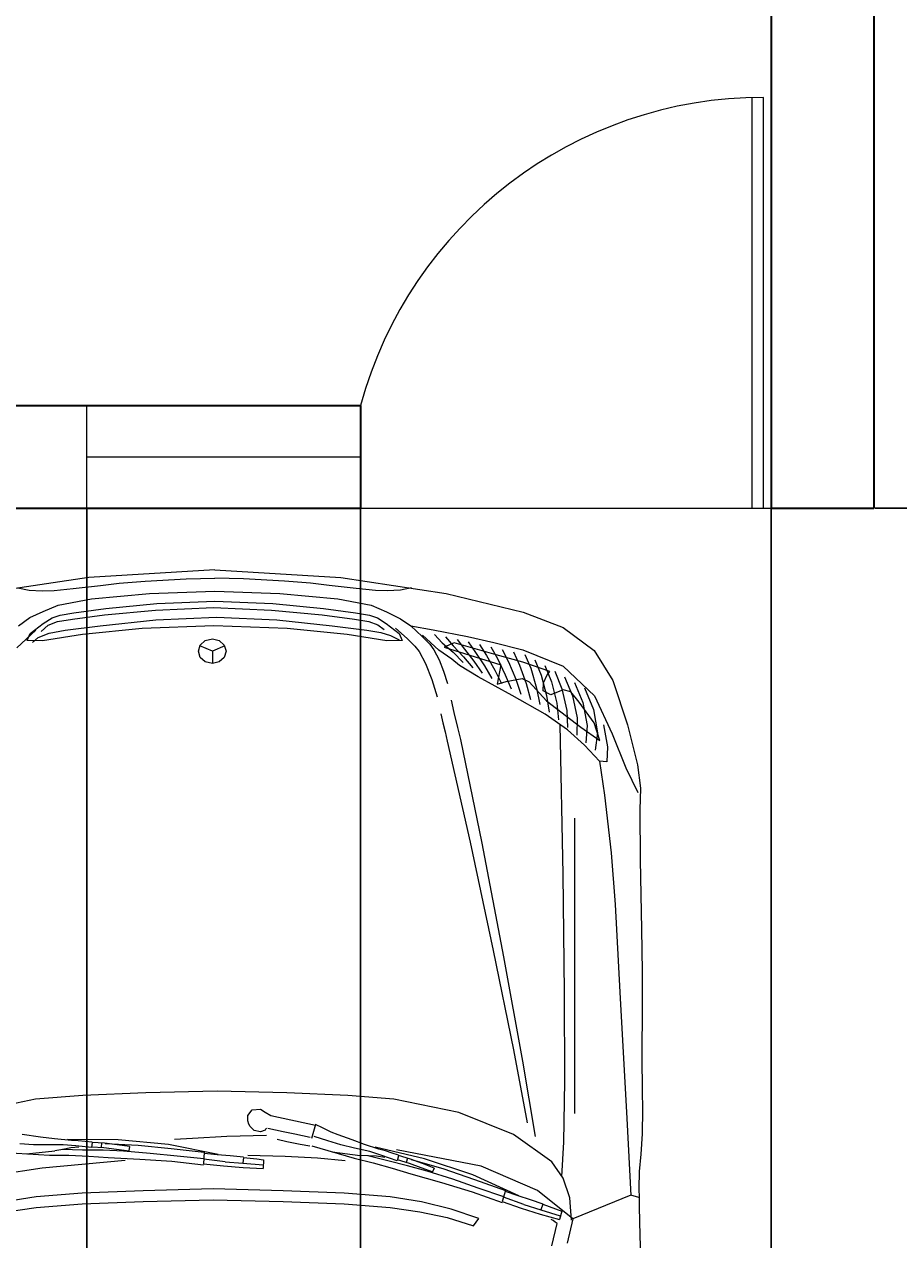
# Model space of a CAD drawing. Units: inches. Extents: x -36 to 401, y -686 to 73.
# Tile 8 of 15: x 248 to 325, y -485 to -379. Entities that reach past the tile are written whole.
import ezdxf

# ---------------------------------------------------------------- set-up
doc = ezdxf.new("R2010")
doc.units = ezdxf.units.IN
doc.header["$MEASUREMENT"] = 0
for name, color, linetype, lineweight in [('A-ANNO-DIMS', 2, 'Continuous', 18), ('A-DOOR', 3, 'Continuous', 18), ('A-GLAZ', 4, 'Continuous', 18), ('A-WALL', 7, 'Continuous', 35), ('C-PKNG-VEHI', 8, 'Continuous', 13)]:
    doc.layers.add(name, color=color, linetype=linetype, lineweight=lineweight)
doc.styles.get("Standard").update_dxf_attribs({"font": 'arial.ttf'})
doc.dimstyles.get("Standard").update_dxf_attribs({"dimtxt": 0.18, "dimasz": 0.18, "dimexe": 0.18, "dimexo": 0.0625, "dimgap": 0.09, "dimtad": 0, "dimtih": 1, "dimtoh": 1, "dimdec": 0, "dimzin": 0, "dimdsep": 46, "dimlunit": 3, "dimtxsty": 'Standard', "dimcen": 0.09, "dimadec": 0, "dimazin": 0, "dimtfac": 1, "dimtdec": 0, "dimtofl": 0, "dimtmove": 0, "dimatfit": 3, "dimfxl": 1, "dimtolj": 1, "dimtzin": 0, "dimarcsym": 0})

# ---------------------------------------------------------------- blocks, each defined once
blk = doc.blocks.new('WIN-24IN')
for p, q in [((0, 9), (24, 9)), ((0, 0), (0, 9)), ((24, 9), (24, 0)), ((0, 4.5), (24, 4.5)), ((24, 0), (0, 0))]:
    blk.add_line(p, q)
blk = doc.blocks.new('*D72')
at = {"layer": 'A-ANNO-DIMS', "color": 0, "lineweight": -2, "transparency": 16777216}
for p, q in [((322.75, -319.21), (401.17, -319.21)), ((400.99, -319.39), (400.99, -370.03)), ((400.99, -421.03), (400.99, -370.39)), ((322.75, -421.21), (401.17, -421.21))]:
    blk.add_line(p, q, dxfattribs=at)
at = {"layer": 'A-ANNO-DIMS', "color": 0, "transparency": 16777216}
for points in [[(400.96, -319.39), (401.02, -319.39), (400.99, -319.21)], [(400.96, -421.03), (401.02, -421.03), (400.99, -421.21)]]:
    blk.add_solid(points, dxfattribs=at)
at = {"layer": 'Defpoints', "color": 0, "transparency": 16777216}
for p in [(322.69, -319.21), (322.69, -421.21), (400.99, -421.21)]:
    blk.add_point(p, dxfattribs=at)
at = {"layer": 'A-ANNO-DIMS', "color": 0, "transparency": 16777216, "insert": (400.99, -370.21), "char_height": 0.18, "attachment_point": 5}
blk.add_mtext('\\A1;8\'-6"', dxfattribs=at)
blk = doc.blocks.new('*D73')
at = {"layer": 'A-ANNO-DIMS', "color": 0, "lineweight": -2, "transparency": 16777216}
for p, q in [((177.19, -421.27), (177.19, -685.69)), ((253.69, -421.27), (253.69, -685.69)), ((177.37, -685.51), (214.9, -685.51)), ((253.51, -685.51), (215.98, -685.51))]:
    blk.add_line(p, q, dxfattribs=at)
at = {"layer": 'A-ANNO-DIMS', "color": 0, "transparency": 16777216}
for points in [[(177.37, -685.48), (177.37, -685.54), (177.19, -685.51)], [(253.51, -685.48), (253.51, -685.54), (253.69, -685.51)]]:
    blk.add_solid(points, dxfattribs=at)
at = {"layer": 'Defpoints', "color": 0, "transparency": 16777216}
for p in [(177.19, -421.21), (253.69, -421.21), (253.69, -685.51)]:
    blk.add_point(p, dxfattribs=at)
at = {"layer": 'A-ANNO-DIMS', "color": 0, "transparency": 16777216, "insert": (215.44, -685.51), "char_height": 0.18, "attachment_point": 5}
blk.add_mtext('\\A1;6\'-4 1/2"', dxfattribs=at)
blk = doc.blocks.new('*D74')
at = {"layer": 'A-ANNO-DIMS', "color": 0, "lineweight": -2, "transparency": 16777216}
for p, q in [((277.69, -412.27), (277.69, -685.69)), ((313.69, -421.27), (313.69, -685.69)), ((277.87, -685.51), (295.36, -685.51)), ((313.51, -685.51), (296.02, -685.51))]:
    blk.add_line(p, q, dxfattribs=at)
at = {"layer": 'A-ANNO-DIMS', "color": 0, "transparency": 16777216}
for points in [[(277.87, -685.48), (277.87, -685.54), (277.69, -685.51)], [(313.51, -685.48), (313.51, -685.54), (313.69, -685.51)]]:
    blk.add_solid(points, dxfattribs=at)
at = {"layer": 'Defpoints', "color": 0, "transparency": 16777216}
for p in [(277.69, -412.21), (313.69, -421.21), (313.69, -685.51)]:
    blk.add_point(p, dxfattribs=at)
at = {"layer": 'A-ANNO-DIMS', "color": 0, "transparency": 16777216, "insert": (295.69, -685.51), "char_height": 0.18, "attachment_point": 5}
blk.add_mtext('\\A1;3\'-0"', dxfattribs=at)

msp = doc.modelspace()

# ---------------------------------------------------------------- linework, layer by layer
at = {"layer": 'A-DOOR'}
for p, q in [((312, -421.21), (312, -385.21)), ((313, -421.21), (313, -385.21)), ((277.69, -421.21), (313.69, -421.21))]:
    msp.add_line(p, q, dxfattribs=at)
msp.add_arc((313, -421.81), 36.6, 90, 164.7978, dxfattribs=at)
at = {"layer": 'A-WALL'}
for p, q in [((313.69, -319.21), (313.69, -421.21)), ((322.69, -319.21), (322.69, -421.21)), ((177.19, -412.21), (277.69, -412.21)), ((277.69, -412.21), (277.69, -421.21)), ((177.19, -421.21), (277.69, -421.21)), ((313.69, -421.21), (322.69, -421.21))]:
    msp.add_line(p, q, dxfattribs=at)
at = {"layer": 'C-PKNG-VEHI'}
for p, q in [((264.9, -426.61), (253.86, -427.27)), ((264.9, -426.61), (275.94, -427.27)), ((253.86, -427.27), (244.61, -428.68)), ((252.5, -428.25), (254.88, -427.98)), ((254.88, -427.98), (256.52, -427.77)), ((256.52, -427.77), (258.79, -427.59)), ((258.79, -427.59), (262.39, -427.41)), ((262.39, -427.41), (264.9, -427.33)), ((267.41, -427.41), (264.9, -427.33)), ((271.01, -427.59), (267.41, -427.41)), ((273.28, -427.77), (271.01, -427.59)), ((274.92, -427.98), (273.28, -427.77)), ((277.29, -428.25), (274.92, -427.98)), ((275.94, -427.27), (285.18, -428.68)), ((247.63, -428.2), (248.62, -428.4)), ((248.62, -428.4), (249.78, -428.46)), ((249.78, -428.46), (250.81, -428.42)), ((250.81, -428.42), (252.5, -428.25)), ((251.17, -429.72), (254.11, -429.14)), ((254.11, -429.14), (259.17, -428.68)), ((259.17, -428.68), (264.9, -428.49)), ((264.9, -428.49), (270.62, -428.68)), ((270.62, -428.68), (275.69, -429.14)), ((275.69, -429.14), (278.62, -429.72)), ((278.98, -428.42), (277.29, -428.25)), ((280.01, -428.46), (278.98, -428.42)), ((281.18, -428.4), (280.01, -428.46)), ((282.16, -428.2), (281.18, -428.4)), ((285.18, -428.68), (291.93, -430.32)), ((249.87, -430.25), (251.17, -429.72)), ((252.55, -430.37), (255.36, -430.01)), ((255.25, -430.56), (259.71, -430.13)), ((255.36, -430.01), (259.82, -429.57)), ((259.71, -430.13), (264.79, -429.91)), ((259.82, -429.57), (264.9, -429.36)), ((264.79, -429.91), (269.87, -430.13)), ((264.9, -429.36), (269.98, -429.57)), ((269.87, -430.13), (274.32, -430.56)), ((269.98, -429.57), (274.43, -430.01)), ((274.43, -430.01), (277.25, -430.37)), ((278.62, -429.72), (279.97, -430.3)), ((247.71, -431.52), (248.7, -430.79)), ((248.7, -430.79), (249.87, -430.25)), ((249.87, -431.31), (250.64, -430.83)), ((250.29, -431.47), (251.11, -431.15)), ((250.64, -430.83), (251.34, -430.57)), ((251.11, -431.15), (252.43, -430.92)), ((251.34, -430.57), (252.55, -430.37)), ((252.43, -430.92), (255.25, -430.56)), ((254.85, -431.51), (259.75, -431)), ((259.75, -431), (265.06, -430.75)), ((265.06, -430.75), (270.35, -431)), ((270.35, -431), (275.2, -431.51)), ((274.32, -430.56), (277.14, -430.92)), ((277.14, -430.92), (278.42, -431.14)), ((277.25, -430.37), (278.46, -430.57)), ((278.42, -431.14), (279.19, -431.42)), ((278.46, -430.57), (279.16, -430.83)), ((279.16, -430.83), (279.92, -431.31)), ((279.97, -430.3), (281.17, -430.9)), ((281.17, -430.9), (282.09, -431.52)), ((291.93, -430.32), (295.45, -431.67)), ((249.22, -431.9), (247.54, -433.43)), ((248.46, -432.81), (248.71, -432.18)), ((248.71, -432.18), (249.87, -431.31)), ((249.41, -432.53), (250.38, -432.17)), ((249.69, -432), (250.29, -431.47)), ((253.3, -432.29), (249.8, -432.82)), ((250.38, -432.17), (251.8, -431.91)), ((251.8, -431.91), (254.85, -431.51)), ((258.55, -431.76), (253.3, -432.29)), ((264.82, -431.52), (258.55, -431.76)), ((271.26, -431.76), (264.82, -431.52)), ((276.52, -432.29), (271.26, -431.76)), ((275.2, -431.51), (278.22, -431.91)), ((279.99, -432.82), (276.52, -432.29)), ((278.22, -431.91), (279.46, -432.11)), ((279.19, -431.42), (279.76, -431.83)), ((279.46, -432.11), (280.32, -432.36)), ((279.92, -431.31), (281.08, -432.18)), ((280.32, -432.36), (281.06, -432.75)), ((280.75, -431.72), (281.76, -432.63)), ((281.08, -432.18), (281.34, -432.81)), ((282.09, -431.52), (283.08, -432.45)), ((282.09, -431.52), (284.06, -431.87)), ((284.55, -433.64), (283.1, -432.32)), ((284.06, -431.87), (287.05, -432.46)), ((284.15, -432.27), (284.84, -433)), ((295.45, -431.67), (298.15, -433.68)), ((249.8, -432.82), (248.46, -432.81)), ((248.91, -432.99), (249.41, -432.53)), ((263.47, -433.74), (263.63, -433.2)), ((264.69, -433.74), (263.59, -433.28)), ((263.63, -433.2), (264.07, -432.81)), ((264.07, -432.81), (264.69, -432.67)), ((264.69, -432.67), (265.3, -432.81)), ((265.78, -433.28), (264.69, -433.74)), ((265.3, -432.81), (265.74, -433.2)), ((265.74, -433.2), (265.91, -433.74)), ((281.34, -432.81), (279.99, -432.82)), ((281.76, -432.63), (282.44, -433.29)), ((282.44, -433.29), (282.81, -433.78)), ((283.08, -432.45), (283.75, -433.12)), ((283.75, -433.12), (284.11, -433.62)), ((284.84, -433), (285.8, -433.83)), ((285.88, -433), (285, -433.39)), ((285, -433.39), (289.99, -434.92)), ((285.14, -432.49), (285.81, -433.28)), ((285.81, -433.28), (286.71, -434.23)), ((289.57, -434.07), (285.88, -433)), ((286.14, -432.7), (286.78, -433.56)), ((287.05, -432.46), (289.38, -432.97)), ((287.13, -432.92), (287.75, -433.84)), ((288.12, -433.14), (288.72, -434.11)), ((289.11, -433.36), (289.69, -434.39)), ((289.38, -432.97), (291.91, -433.61)), ((263.63, -434.28), (263.47, -433.74)), ((264.07, -434.67), (263.63, -434.28)), ((264.69, -433.74), (264.69, -434.82)), ((265.74, -434.28), (265.3, -434.67)), ((265.91, -433.74), (265.74, -434.28)), ((282.81, -433.78), (283.37, -434.81)), ((284.11, -433.62), (284.57, -434.49)), ((285.67, -434.44), (284.55, -433.64)), ((284.57, -434.49), (284.96, -435.48)), ((286.35, -434.99), (285.67, -434.44)), ((285.8, -433.83), (286.67, -434.74)), ((286.71, -434.23), (287.51, -435.2)), ((286.78, -433.56), (287.62, -434.62)), ((287.75, -433.84), (288.54, -435.01)), ((288.72, -434.11), (289.45, -435.41)), ((290.21, -434.23), (289.57, -434.07)), ((289.69, -434.39), (290.36, -435.8)), ((290.11, -433.58), (290.66, -434.67)), ((291.9, -434.7), (290.21, -434.23)), ((291.1, -433.8), (291.63, -434.95)), ((291.91, -433.61), (295.43, -435.05)), ((292.09, -434.02), (292.6, -435.23)), ((298.15, -433.68), (299.81, -436.32)), ((264.69, -434.82), (264.07, -434.67)), ((265.3, -434.67), (264.69, -434.82)), ((283.37, -434.81), (283.94, -436.21)), ((284.96, -435.48), (285.31, -436.57)), ((287.98, -436), (286.35, -434.99)), ((287.62, -434.62), (288.35, -435.66)), ((288.54, -435.01), (289.19, -436.12)), ((289.45, -435.41), (290.04, -436.58)), ((289.99, -434.92), (289.66, -436.62)), ((290.66, -434.67), (291.28, -436.19)), ((291.63, -434.95), (292.19, -436.58)), ((294.27, -435.51), (291.9, -434.7)), ((292.6, -435.23), (293.1, -436.98)), ((292.96, -434.51), (293.51, -435.83)), ((293.83, -435), (294.43, -436.43)), ((294.05, -435.81), (294.27, -435.51)), ((294.7, -435.49), (295.34, -437.04)), ((295.43, -435.05), (298.2, -437.66)), ((283.94, -436.21), (284.4, -437.75)), ((290.98, -437.62), (287.98, -436)), ((289.66, -436.62), (290.44, -436.4)), ((290.36, -435.8), (290.88, -437.04)), ((290.44, -436.4), (291.84, -436.13)), ((291.28, -436.19), (291.72, -437.5)), ((291.84, -436.13), (292.47, -436.42)), ((292.19, -436.58), (292.57, -437.96)), ((292.47, -436.42), (293.98, -438.1)), ((293.51, -435.83), (293.99, -437.63)), ((293.68, -437.21), (293.71, -436.5)), ((293.71, -436.5), (294.05, -435.81)), ((294.43, -436.43), (294.88, -438.28)), ((295.57, -435.98), (296.26, -437.64)), ((296.44, -436.47), (297.18, -438.24)), ((299.81, -436.32), (301.08, -440.19)), ((293.86, -439.25), (290.98, -437.62)), ((293.1, -436.98), (293.41, -438.42)), ((294.36, -437.55), (293.68, -437.21)), ((293.99, -437.63), (294.22, -439.08)), ((295.43, -437.13), (294.36, -437.55)), ((295.34, -437.04), (295.77, -438.93)), ((296.12, -437.31), (295.43, -437.13)), ((296.86, -438.2), (296.12, -437.31)), ((296.26, -437.64), (296.66, -439.59)), ((297.31, -436.96), (298.09, -438.84)), ((298.2, -437.66), (299.75, -440.98)), ((285.62, -438.03), (285.87, -439.1)), ((293.98, -438.1), (297, -440.39)), ((294.88, -438.28), (295.02, -439.75)), ((298.17, -440.03), (296.86, -438.2)), ((297.18, -438.24), (297.55, -440.24)), ((284.72, -439.22), (284.9, -440.02)), ((285.87, -439.1), (286.19, -440.42)), ((295.82, -440.64), (293.86, -439.25)), ((295.77, -438.93), (295.83, -440.42)), ((296.66, -439.59), (296.63, -441.09)), ((298.09, -438.84), (298.44, -440.89)), ((284.9, -440.02), (285.09, -440.81)), ((285.09, -440.81), (285.28, -441.61)), ((286.19, -440.42), (286.44, -441.49)), ((295.16, -440.19), (295.41, -453.27)), ((297.3, -441.98), (295.82, -440.64)), ((297, -440.39), (298.65, -441.55)), ((297.55, -440.24), (297.44, -441.76)), ((298.65, -441.55), (298.17, -440.03)), ((298.97, -440.2), (299.34, -442.12)), ((301.08, -440.19), (301.96, -443.71)), ((285.28, -441.61), (287.29, -450.46)), ((286.44, -441.49), (288.32, -450.56)), ((298.44, -440.89), (298.24, -442.42)), ((299.75, -440.98), (300.95, -443.97)), ((298.63, -443.37), (297.3, -441.98)), ((299.34, -442.12), (299.28, -443.44)), ((298.63, -443.37), (299.08, -446.35)), ((299.28, -443.44), (298.63, -443.37)), ((300.95, -443.97), (301.98, -446.13)), ((301.96, -443.71), (302.21, -445.75)), ((302.21, -445.75), (302.17, -447.63)), ((299.08, -446.35), (299.65, -451.41)), ((302.17, -447.63), (302.19, -452.04)), ((296.48, -474.24), (296.48, -448.37)), ((287.29, -450.46), (289.32, -459.97)), ((288.32, -450.56), (290.22, -460.51)), ((299.65, -451.41), (300, -455.94)), ((302.19, -452.04), (302.31, -458.1)), ((295.41, -453.27), (295.53, -463.63)), ((300, -455.94), (300.4, -463.61)), ((302.31, -458.1), (302.38, -461.79)), ((289.32, -459.97), (291.08, -468.67)), ((290.22, -460.51), (291.87, -469.65)), ((302.38, -461.79), (302.37, -464.78)), ((295.53, -463.63), (295.56, -471.41)), ((300.4, -463.61), (301.02, -474.68)), ((302.37, -464.78), (302.35, -469.32)), ((291.08, -468.67), (292.29, -475.07)), ((302.35, -469.32), (302.38, -472.26)), ((291.87, -469.65), (292.99, -476.26)), ((295.56, -471.41), (295.48, -476.75)), ((253.33, -472.66), (249.19, -472.98)), ((258.85, -472.45), (253.33, -472.66)), ((265.1, -472.29), (258.85, -472.45)), ((271.23, -472.45), (265.1, -472.29)), ((276.57, -472.66), (271.23, -472.45)), ((280.61, -472.98), (276.57, -472.66)), ((302.38, -472.26), (302.41, -473.9)), ((249.19, -472.98), (243.51, -474.17)), ((268.18, -473.93), (268.91, -473.86)), ((268.91, -473.86), (269.32, -474.14)), ((286.29, -474.17), (280.61, -472.98)), ((302.41, -473.9), (302.36, -476.04)), ((267.8, -474.89), (267.81, -474.42)), ((267.89, -475.19), (267.8, -474.89)), ((267.81, -474.42), (268.18, -473.93)), ((269.32, -474.14), (269.82, -474.41)), ((269.82, -474.41), (273.72, -475.28)), ((291.09, -476.09), (286.29, -474.17)), ((301.02, -474.68), (301.37, -481.43)), ((268.01, -475.38), (267.89, -475.19)), ((268.35, -475.73), (268.01, -475.38)), ((268.92, -475.85), (268.35, -475.73)), ((269.32, -475.72), (268.92, -475.85)), ((269.38, -475.6), (269.32, -475.72)), ((269.45, -475.55), (269.38, -475.6)), ((270.91, -475.85), (269.56, -475.57)), ((271.92, -476.07), (270.91, -475.85)), ((273.74, -475.22), (273.38, -476.44)), ((274.35, -475.5), (273.74, -475.22)), ((275.1, -475.87), (274.35, -475.5)), ((275.72, -476.13), (275.1, -475.87)), ((249, -476.99), (247.8, -476.91)), ((249.63, -476.32), (248.02, -476.1)), ((250.25, -477), (249, -476.99)), ((250.84, -476.48), (249.63, -476.32)), ((251.61, -477), (250.25, -477)), ((252.34, -476.61), (250.84, -476.48)), ((252.72, -477.09), (251.61, -477)), ((256.43, -476.56), (251.99, -476.52)), ((252.94, -476.65), (252.34, -476.61)), ((254.11, -477.24), (252.72, -477.09)), ((253.55, -476.71), (252.94, -476.65)), ((254.15, -476.75), (253.55, -476.71)), ((254.16, -476.79), (254.11, -477.24)), ((255.23, -476.85), (254.13, -476.78)), ((254.98, -476.83), (254.94, -477.22)), ((256.34, -476.99), (255.23, -476.85)), ((255.3, -476.88), (258.2, -477.02)), ((257.43, -477.14), (256.34, -476.99)), ((260.85, -476.95), (256.43, -476.56)), ((258.2, -477.02), (261.09, -477.32)), ((265.21, -477.83), (260.85, -476.95)), ((262.96, -476.44), (261.37, -476.52)), ((265.96, -476.27), (262.96, -476.44)), ((269.44, -476.17), (265.96, -476.27)), ((270.36, -476.5), (271.22, -476.7)), ((271.22, -476.7), (272.39, -476.93)), ((273.27, -476.36), (271.92, -476.07)), ((272.39, -476.93), (273.23, -477.07)), ((274.8, -476.63), (273.61, -476.27)), ((275.95, -476.98), (274.8, -476.63)), ((276.96, -476.55), (275.72, -476.13)), ((277.16, -477.27), (275.95, -476.98)), ((278.03, -476.96), (276.96, -476.55)), ((279.29, -477.36), (278.03, -476.96)), ((294.44, -478.47), (291.09, -476.09)), ((295.48, -476.75), (295.31, -479.77)), ((302.36, -476.04), (302.24, -477.82)), ((246.55, -477.67), (250.4, -477.89)), ((248.39, -477.77), (250.88, -477.53)), ((250.4, -477.89), (252.12, -477.91)), ((251.58, -477.4), (250.88, -477.53)), ((253.32, -477.45), (251.54, -477.4)), ((252.29, -477.26), (251.58, -477.4)), ((252.12, -477.91), (253.85, -477.99)), ((253, -477.21), (252.29, -477.26)), ((255.11, -477.47), (253.32, -477.45)), ((253.85, -477.99), (255.56, -478.1)), ((254.09, -477.16), (255.19, -477.24)), ((256.9, -477.54), (255.11, -477.47)), ((255.19, -477.24), (256.3, -477.36)), ((255.56, -478.1), (258.34, -478.24)), ((256.3, -477.36), (257.39, -477.51)), ((259.25, -477.74), (256.9, -477.54)), ((257.43, -477.14), (257.37, -477.51)), ((261.6, -477.99), (259.25, -477.74)), ((261.09, -477.32), (263.97, -477.64)), ((263.94, -478.23), (261.6, -477.99)), ((263.97, -477.64), (263.92, -478.65)), ((263.97, -477.72), (265.12, -477.84)), ((265.12, -477.84), (266.26, -477.94)), ((266.26, -477.94), (267.41, -478.05)), ((267.42, -478.09), (267.37, -478.61)), ((267.42, -478.09), (268.01, -478.16)), ((271.06, -478), (267.81, -477.94)), ((273.92, -478.16), (271.06, -478)), ((273.41, -477.09), (277.11, -478.17)), ((275.18, -477.6), (277.66, -477.93)), ((278.5, -477.58), (277.16, -477.27)), ((278.38, -477.96), (277.66, -477.93)), ((280.06, -478.4), (278.33, -477.95)), ((279.09, -477.98), (278.38, -477.96)), ((279.56, -477.92), (278.5, -477.58)), ((283.29, -478.23), (278.96, -477.2)), ((279.8, -478.09), (279.09, -477.98)), ((279.87, -477.53), (279.29, -477.36)), ((280.88, -478.38), (279.56, -477.92)), ((280.45, -477.73), (279.87, -477.53)), ((281.02, -477.91), (280.45, -477.73)), ((288.25, -478.87), (280.83, -477.43)), ((281.02, -477.95), (280.88, -478.38)), ((282.06, -478.24), (281, -477.93)), ((302.24, -477.82), (302.12, -479.33)), ((249.77, -479.03), (245.92, -479.63)), ((257.06, -478.36), (249.77, -479.03)), ((258.34, -478.24), (261.15, -478.43)), ((261.15, -478.43), (263.91, -478.74)), ((263.92, -478.65), (265.66, -478.84)), ((265.82, -478.48), (263.93, -478.25)), ((265.66, -478.84), (267.4, -478.98)), ((265.82, -478.48), (267.37, -478.61)), ((267.37, -478.61), (269.15, -478.74)), ((267.4, -478.98), (269.15, -479.07)), ((268.01, -478.16), (268.6, -478.23)), ((268.6, -478.23), (269.18, -478.31)), ((269.18, -478.31), (269.15, -479.07)), ((276.34, -478.4), (273.92, -478.16)), ((277.11, -478.17), (278.78, -478.57)), ((278.78, -478.57), (280.45, -479.05)), ((281.8, -478.82), (280.06, -478.4)), ((280.45, -479.05), (282.1, -479.53)), ((280.88, -478.29), (281.93, -478.61)), ((281.81, -478.17), (281.69, -478.54)), ((283.52, -479.29), (281.8, -478.82)), ((281.93, -478.61), (282.98, -478.98)), ((283.1, -478.63), (282.06, -478.24)), ((282.12, -478.29), (284.9, -479.07)), ((282.98, -478.98), (284.01, -479.37)), ((284.13, -479.03), (283.1, -478.63)), ((287.51, -479.61), (283.29, -478.23)), ((284.13, -479.03), (283.99, -479.37)), ((284.9, -479.07), (287.66, -480.02)), ((293.18, -481), (288.25, -478.87)), ((295.45, -479.91), (294.44, -478.47)), ((282.1, -479.53), (284.77, -480.3)), ((285.77, -480.01), (283.52, -479.29)), ((288, -480.79), (285.77, -480.01)), ((291.55, -481.45), (287.51, -479.61)), ((287.66, -480.02), (290.39, -480.98)), ((296.04, -481.65), (295.45, -479.91)), ((302.12, -479.33), (302.07, -480.82)), ((253.29, -481.23), (249.25, -481.55)), ((258.62, -481.02), (253.29, -481.23)), ((264.76, -480.86), (258.62, -481.02)), ((270.9, -481.02), (264.76, -480.86)), ((276.24, -481.23), (270.9, -481.02)), ((280.27, -481.55), (276.24, -481.23)), ((284.77, -480.3), (287.47, -481.11)), ((287.47, -481.11), (290.09, -482.04)), ((290.23, -481.55), (288, -480.79)), ((290.39, -480.98), (290.11, -481.96)), ((290.37, -481.06), (291.46, -481.43)), ((296.28, -483.48), (293.18, -481)), ((302.07, -480.82), (302.1, -481.65)), ((249.25, -481.55), (246.51, -481.99)), ((249.25, -482.49), (253.29, -482.17)), ((253.29, -482.17), (258.62, -481.96)), ((258.62, -481.96), (264.76, -481.8)), ((264.76, -481.8), (270.9, -481.96)), ((270.9, -481.96), (276.24, -482.17)), ((276.24, -482.17), (280.27, -482.49)), ((283.01, -481.99), (280.27, -481.55)), ((285.63, -482.64), (283.01, -481.99)), ((290.11, -481.96), (291.77, -482.53)), ((292, -482.22), (290.21, -481.57)), ((291.46, -481.43), (292.56, -481.79)), ((292, -482.22), (293.49, -482.69)), ((292.56, -481.79), (293.65, -482.16)), ((293.65, -482.2), (293.49, -482.69)), ((293.65, -482.2), (294.21, -482.39)), ((294.21, -482.39), (294.77, -482.6)), ((296.17, -483.6), (296.04, -481.65)), ((301.37, -481.39), (296.28, -483.48)), ((302.09, -481.61), (301.37, -481.39)), ((302.1, -481.65), (302.11, -482.43)), ((246.64, -482.86), (249.25, -482.49)), ((280.27, -482.49), (282.89, -482.86)), ((282.89, -482.86), (285.26, -483.36)), ((285.26, -483.36), (287.57, -484.08)), ((288.06, -483.44), (285.63, -482.64)), ((287.57, -484.08), (288.06, -483.44)), ((291.77, -482.53), (293.43, -483.06)), ((293.43, -483.06), (295.11, -483.54)), ((293.49, -482.69), (295.19, -483.22)), ((294.77, -482.6), (295.32, -482.81)), ((295.32, -482.81), (295.11, -483.54)), ((296.28, -483.48), (295.79, -485.61)), ((302.11, -482.43), (302.16, -484.94)), ((294.57, -483.63), (294.4, -483.52)), ((294.45, -485.83), (294.91, -483.89)), ((294.74, -483.76), (294.57, -483.63)), ((294.91, -483.89), (294.74, -483.76)), ((302.16, -484.94), (302.3, -489.38))]:
    msp.add_line(p, q, dxfattribs=at)

# ---------------------------------------------------------------- block references
at = {"layer": 'A-GLAZ'}
msp.add_blockref('WIN-24IN', (253.69, -421.21), dxfattribs=at)

# ---------------------------------------------------------------- dimensions: what is measured, and where the dimension line sits
at = {"layer": 'A-ANNO-DIMS'}
dim = msp.add_linear_dim(base=(400.99, -421.21), p1=(322.69, -319.21), p2=(322.69, -421.21), angle=90, dimstyle='Standard', override={"dimdec": 1, "dimlfac": 1, "dimrnd": 0, "dimzin": 1, "dimdsep": 46, "dimlunit": 4, "dimfrac": 2}, dxfattribs=at)
dim.commit()
dim.dimension.update_dxf_attribs({"geometry": '*D72', "text_midpoint": (400.99, -370.21)})
for base, p1, p2, picture, middle in [((313.69, -685.51), (277.69, -412.21), (313.69, -421.21), '*D74', (295.69, -685.51)), ((253.69, -685.51), (177.19, -421.21), (253.69, -421.21), '*D73', (215.44, -685.51))]:
    dim = msp.add_linear_dim(base=base, p1=p1, p2=p2, dimstyle='Standard', override={"dimdec": 1, "dimlfac": 1, "dimrnd": 0, "dimzin": 1, "dimdsep": 46, "dimlunit": 4, "dimfrac": 2}, dxfattribs=at)
    dim.commit()
    dim.dimension.update_dxf_attribs({"geometry": picture, "text_midpoint": middle})

doc.saveas('drawing.dxf')
